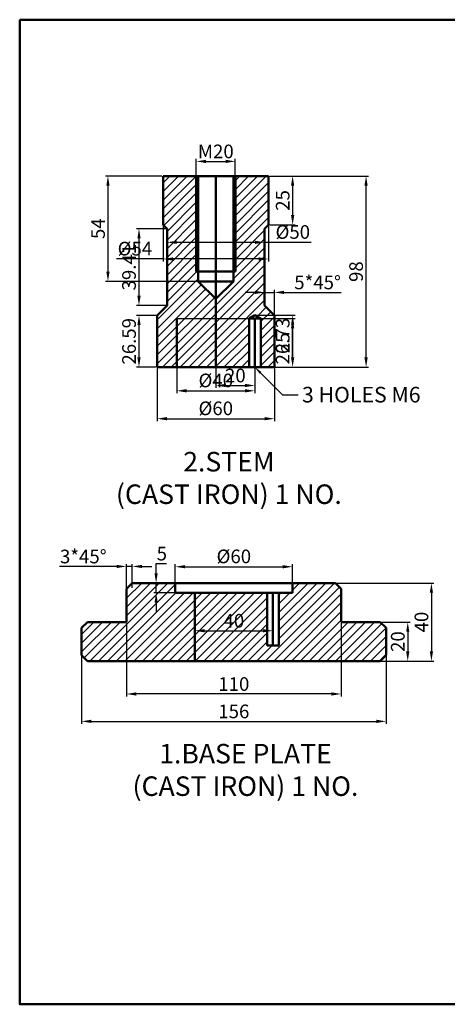
# Model space of a CAD drawing. Units: millimetres. Extents: x 51 to 972, y -225 to 280.
# Tile 1 of 3: x 51 to 270, y -225 to 280. Entities that reach past the tile are written whole.
import ezdxf
from ezdxf import colors
from ezdxf.entities.mleader import LeaderData, LeaderLine
from ezdxf.math import Vec2, Vec3

# ---------------------------------------------------------------- set-up
doc = ezdxf.new("R2010")
doc.units = ezdxf.units.MM
doc.header["$LTSCALE"] = 0.5
for name, color, linetype, lineweight in [('M-DIMS', 2, 'Continuous', 25), ('M-HATC', 8, 'Continuous', 18), ('M-OUTL', 7, 'Continuous', 50), ('M-TEXT', 7, 'Continuous', 25), ('M-TTLB', 7, 'Continuous', 50)]:
    doc.layers.add(name, color=color, linetype=linetype, lineweight=lineweight)
doc.styles.get("Standard").update_dxf_attribs({"font": 'arial.ttf'})
doc.dimstyles.new('ISO-25', dxfattribs={"dimtxt": 7, "dimasz": 5, "dimexe": 1.25, "dimexo": 0.625, "dimtad": 1, "dimtoh": 1, "dimtxsty": 'Standard', "dimcen": 2.5, "dimadec": 0, "dimazin": 0, "dimtfac": 1, "dimtmove": 0, "dimatfit": 3, "dimfxl": 1, "dimarcsym": 0})

# ---------------------------------------------------------------- blocks, each defined once
blk = doc.blocks.new('*D1')
at = {"layer": 'Defpoints', "color": 0, "transparency": 16777216}
for p in [(121.33, 101.59), (181.33, 101.59), (181.33, 75.2)]:
    blk.add_point(p, dxfattribs=at)
at = {"layer": 'M-DIMS', "color": 0, "lineweight": -2, "transparency": 16777216}
for p, q in [((121.33, 100.96), (121.33, 73.95)), ((181.33, 100.96), (181.33, 73.95)), ((126.33, 75.2), (176.33, 75.2))]:
    blk.add_line(p, q, dxfattribs=at)
at = {"layer": 'M-DIMS', "color": 0, "transparency": 16777216}
for points in [[(126.33, 76.04), (126.33, 74.37), (121.33, 75.2)], [(176.33, 76.04), (176.33, 74.37), (181.33, 75.2)]]:
    blk.add_solid(points, dxfattribs=at)
at = {"layer": 'M-DIMS', "color": 0, "transparency": 16777216, "insert": (151.33, 79.6), "char_height": 7, "attachment_point": 5}
blk.add_mtext('%%C60', dxfattribs=at)
blk = doc.blocks.new('*D2')
at = {"layer": 'Defpoints', "color": 0, "transparency": 16777216}
for p in [(131.33, 101.59), (171.33, 101.59), (171.33, 89.5)]:
    blk.add_point(p, dxfattribs=at)
at = {"layer": 'M-DIMS', "color": 0, "lineweight": -2, "transparency": 16777216}
for p, q in [((131.33, 100.96), (131.33, 88.25)), ((171.33, 100.96), (171.33, 88.25)), ((136.33, 89.5), (166.33, 89.5))]:
    blk.add_line(p, q, dxfattribs=at)
at = {"layer": 'M-DIMS', "color": 0, "transparency": 16777216}
for points in [[(136.33, 90.34), (136.33, 88.67), (131.33, 89.5)], [(166.33, 90.34), (166.33, 88.67), (171.33, 89.5)]]:
    blk.add_solid(points, dxfattribs=at)
at = {"layer": 'M-DIMS', "color": 0, "transparency": 16777216, "insert": (151.33, 93.9), "char_height": 7, "attachment_point": 5}
blk.add_mtext('%%C40', dxfattribs=at)
blk = doc.blocks.new('*D3')
at = {"layer": 'Defpoints', "color": 0, "transparency": 16777216}
for p in [(126.33, 168.2), (176.33, 168.2), (176.33, 165.61)]:
    blk.add_point(p, dxfattribs=at)
at = {"layer": 'M-DIMS', "color": 0, "lineweight": -2, "transparency": 16777216}
for p, q in [((126.33, 167.58), (126.33, 164.36)), ((176.33, 167.58), (176.33, 164.36)), ((131.33, 165.61), (171.33, 165.61)), ((176.33, 165.61), (200.2, 165.61))]:
    blk.add_line(p, q, dxfattribs=at)
at = {"layer": 'M-DIMS', "color": 0, "transparency": 16777216}
for points in [[(131.33, 166.44), (131.33, 164.77), (126.33, 165.61)], [(171.33, 166.44), (171.33, 164.77), (176.33, 165.61)]]:
    blk.add_solid(points, dxfattribs=at)
at = {"layer": 'M-DIMS', "color": 0, "transparency": 16777216, "insert": (190.77, 170), "char_height": 7, "attachment_point": 5}
blk.add_mtext('%%C50', dxfattribs=at)
blk = doc.blocks.new('*D4')
at = {"layer": 'Defpoints', "color": 0, "transparency": 16777216}
for p in [(124.33, 187.09), (178.33, 187.09), (178.33, 157.07)]:
    blk.add_point(p, dxfattribs=at)
at = {"layer": 'M-DIMS', "color": 0, "lineweight": -2, "transparency": 16777216}
for p, q in [((124.33, 186.46), (124.33, 155.82)), ((178.33, 186.46), (178.33, 155.82)), ((124.33, 157.07), (100.47, 157.07)), ((173.33, 157.07), (129.33, 157.07))]:
    blk.add_line(p, q, dxfattribs=at)
at = {"layer": 'M-DIMS', "color": 0, "transparency": 16777216}
for points in [[(129.33, 157.9), (129.33, 156.23), (124.33, 157.07)], [(173.33, 157.9), (173.33, 156.23), (178.33, 157.07)]]:
    blk.add_solid(points, dxfattribs=at)
at = {"layer": 'M-DIMS', "color": 0, "transparency": 16777216, "insert": (109.9, 161.46), "char_height": 7, "attachment_point": 5}
blk.add_mtext('%%C54', dxfattribs=at)
blk = doc.blocks.new('*D5')
at = {"layer": 'Defpoints', "color": 0, "transparency": 16777216}
for p in [(161.33, 207.09), (141.33, 199.59), (161.33, 199.59)]:
    blk.add_point(p, dxfattribs=at)
at = {"layer": 'M-DIMS', "color": 0, "lineweight": -2, "transparency": 16777216}
for p, q in [((141.33, 200.21), (141.33, 208.34)), ((146.33, 207.09), (156.33, 207.09)), ((161.33, 200.21), (161.33, 208.34))]:
    blk.add_line(p, q, dxfattribs=at)
at = {"layer": 'M-DIMS', "color": 0, "transparency": 16777216}
for points in [[(146.33, 207.92), (146.33, 206.25), (141.33, 207.09)], [(156.33, 207.92), (156.33, 206.25), (161.33, 207.09)]]:
    blk.add_solid(points, dxfattribs=at)
at = {"layer": 'M-DIMS', "color": 0, "transparency": 16777216, "insert": (151.33, 211.29), "char_height": 7, "attachment_point": 5}
blk.add_mtext('M20', dxfattribs=at)
blk = doc.blocks.new('*D6')
at = {"layer": 'Defpoints', "color": 0, "transparency": 16777216}
for p in [(181.33, 139.95), (176.33, 133.18), (181.33, 128.18)]:
    blk.add_point(p, dxfattribs=at)
at = {"layer": 'M-DIMS', "color": 0, "lineweight": -2, "transparency": 16777216}
for p, q in [((171.33, 139.95), (166.33, 139.95)), ((176.33, 133.8), (176.33, 141.2)), ((176.33, 139.95), (181.33, 139.95)), ((181.33, 128.8), (181.33, 141.2)), ((186.33, 139.95), (215.56, 139.95))]:
    blk.add_line(p, q, dxfattribs=at)
at = {"layer": 'M-DIMS', "color": 0, "transparency": 16777216}
for points in [[(171.33, 140.78), (171.33, 139.12), (176.33, 139.95)], [(186.33, 140.78), (186.33, 139.12), (181.33, 139.95)]]:
    blk.add_solid(points, dxfattribs=at)
at = {"layer": 'M-DIMS', "color": 0, "transparency": 16777216, "insert": (203.45, 144.14), "char_height": 7, "attachment_point": 5}
blk.add_mtext('5*45%%D', dxfattribs=at)
blk = doc.blocks.new('*D7')
at = {"layer": 'Defpoints', "color": 0, "transparency": 16777216}
for p in [(178.33, 199.59), (228.3, 199.59), (181.45, 101.59)]:
    blk.add_point(p, dxfattribs=at)
at = {"layer": 'M-DIMS', "color": 0, "lineweight": -2, "transparency": 16777216}
for p, q in [((178.96, 199.59), (229.55, 199.59)), ((228.3, 106.59), (228.3, 194.59)), ((182.08, 101.59), (229.55, 101.59))]:
    blk.add_line(p, q, dxfattribs=at)
at = {"layer": 'M-DIMS', "color": 0, "transparency": 16777216}
for points in [[(227.46, 194.59), (229.13, 194.59), (228.3, 199.59)], [(227.46, 106.59), (229.13, 106.59), (228.3, 101.59)]]:
    blk.add_solid(points, dxfattribs=at)
at = {"layer": 'M-DIMS', "color": 0, "transparency": 16777216, "insert": (224.1, 150.59), "char_height": 7, "attachment_point": 5, "rotation": 90}
blk.add_mtext('98', dxfattribs=at)
blk = doc.blocks.new('*D8')
at = {"layer": 'Defpoints', "color": 0, "transparency": 16777216}
for p in [(124.33, 199.59), (96.09, 145.59), (151.33, 145.59)]:
    blk.add_point(p, dxfattribs=at)
at = {"layer": 'M-DIMS', "color": 0, "lineweight": -2, "transparency": 16777216}
for p, q in [((123.71, 199.59), (94.84, 199.59)), ((96.09, 194.59), (96.09, 150.59)), ((150.71, 145.59), (94.84, 145.59))]:
    blk.add_line(p, q, dxfattribs=at)
at = {"layer": 'M-DIMS', "color": 0, "transparency": 16777216}
for points in [[(95.26, 194.59), (96.93, 194.59), (96.09, 199.59)], [(95.26, 150.59), (96.93, 150.59), (96.09, 145.59)]]:
    blk.add_solid(points, dxfattribs=at)
at = {"layer": 'M-DIMS', "color": 0, "transparency": 16777216, "insert": (91.91, 172.59), "char_height": 7, "attachment_point": 5, "rotation": 90}
blk.add_mtext('54', dxfattribs=at)
blk = doc.blocks.new('*D20')
at = {"layer": 'Defpoints', "color": 0, "ltscale": 0.5, "transparency": 16777216}
for p in [(82.57, -39.05), (238.57, -39.05), (238.57, -79.94)]:
    blk.add_point(p, dxfattribs=at)
at = {"layer": 'M-DIMS', "color": 0, "lineweight": -2, "ltscale": 0.5, "transparency": 16777216}
for p, q in [((82.57, -39.67), (82.57, -81.19)), ((238.57, -39.67), (238.57, -81.19)), ((87.57, -79.94), (233.57, -79.94))]:
    blk.add_line(p, q, dxfattribs=at)
at = {"layer": 'M-DIMS', "color": 0, "ltscale": 0.5, "transparency": 16777216}
for points in [[(87.57, -79.1), (87.57, -80.77), (82.57, -79.94)], [(233.57, -79.1), (233.57, -80.77), (238.57, -79.94)]]:
    blk.add_solid(points, dxfattribs=at)
at = {"layer": 'M-DIMS', "color": 0, "ltscale": 0.5, "transparency": 16777216, "insert": (160.57, -75.74), "char_height": 7, "attachment_point": 5}
blk.add_mtext('156', dxfattribs=at)
blk = doc.blocks.new('*D21')
at = {"layer": 'Defpoints', "color": 0, "ltscale": 0.5, "transparency": 16777216}
for p in [(105.57, -29.05), (215.57, -29.05), (105.57, -65.91)]:
    blk.add_point(p, dxfattribs=at)
at = {"layer": 'M-DIMS', "color": 0, "lineweight": -2, "ltscale": 0.5, "transparency": 16777216}
for p, q in [((105.57, -29.67), (105.57, -67.16)), ((215.57, -29.67), (215.57, -67.16)), ((210.57, -65.91), (110.57, -65.91))]:
    blk.add_line(p, q, dxfattribs=at)
at = {"layer": 'M-DIMS', "color": 0, "ltscale": 0.5, "transparency": 16777216}
for points in [[(110.57, -65.07), (110.57, -66.74), (105.57, -65.91)], [(210.57, -65.07), (210.57, -66.74), (215.57, -65.91)]]:
    blk.add_solid(points, dxfattribs=at)
at = {"layer": 'M-DIMS', "color": 0, "ltscale": 0.5, "transparency": 16777216, "insert": (160.57, -61.71), "char_height": 7, "attachment_point": 5}
blk.add_mtext('110', dxfattribs=at)
blk = doc.blocks.new('*D22')
at = {"layer": 'Defpoints', "color": 0, "ltscale": 0.5, "transparency": 16777216}
for p in [(190.57, -0.69), (130.57, -9.05), (190.57, -9.05)]:
    blk.add_point(p, dxfattribs=at)
at = {"layer": 'M-DIMS', "color": 0, "lineweight": -2, "ltscale": 0.5, "transparency": 16777216}
for p, q in [((130.57, -8.42), (130.57, 0.56)), ((190.57, -8.42), (190.57, 0.56)), ((135.57, -0.69), (185.57, -0.69))]:
    blk.add_line(p, q, dxfattribs=at)
at = {"layer": 'M-DIMS', "color": 0, "ltscale": 0.5, "transparency": 16777216}
for points in [[(135.57, 0.14), (135.57, -1.52), (130.57, -0.69)], [(185.57, 0.14), (185.57, -1.52), (190.57, -0.69)]]:
    blk.add_solid(points, dxfattribs=at)
at = {"layer": 'M-DIMS', "color": 0, "ltscale": 0.5, "transparency": 16777216, "insert": (160.57, 3.71), "char_height": 7, "attachment_point": 5}
blk.add_mtext('%%C60', dxfattribs=at)
blk = doc.blocks.new('*D23')
at = {"layer": 'Defpoints', "color": 0, "ltscale": 0.5, "transparency": 16777216}
for p in [(140.57, -31.55), (180.57, -31.55), (180.57, -33.49)]:
    blk.add_point(p, dxfattribs=at)
at = {"layer": 'M-DIMS', "color": 0, "lineweight": -2, "ltscale": 0.5, "transparency": 16777216}
for p, q in [((140.57, -32.17), (140.57, -34.74)), ((145.57, -33.49), (175.57, -33.49)), ((180.57, -32.17), (180.57, -34.74))]:
    blk.add_line(p, q, dxfattribs=at)
at = {"layer": 'M-DIMS', "color": 0, "ltscale": 0.5, "transparency": 16777216}
for points in [[(145.57, -32.66), (145.57, -34.33), (140.57, -33.49)], [(175.57, -32.66), (175.57, -34.33), (180.57, -33.49)]]:
    blk.add_solid(points, dxfattribs=at)
at = {"layer": 'M-DIMS', "color": 0, "ltscale": 0.5, "transparency": 16777216, "insert": (160.57, -29.29), "char_height": 7, "attachment_point": 5}
blk.add_mtext('40', dxfattribs=at)
blk = doc.blocks.new('*D24')
at = {"layer": 'Defpoints', "color": 0, "ltscale": 0.5, "transparency": 16777216}
for p in [(130.57, -9.05), (120.76, -14.05), (130.57, -14.05)]:
    blk.add_point(p, dxfattribs=at)
at = {"layer": 'M-DIMS', "color": 0, "lineweight": -2, "ltscale": 0.5, "transparency": 16777216}
for p, q in [((120.76, -4.05), (120.76, 0.95)), ((120.76, 0.95), (126.03, 0.95)), ((129.94, -9.05), (119.51, -9.05)), ((120.76, -14.05), (120.76, -9.05)), ((129.94, -14.05), (119.51, -14.05)), ((120.76, -19.05), (120.76, -24.05))]:
    blk.add_line(p, q, dxfattribs=at)
at = {"layer": 'M-DIMS', "color": 0, "ltscale": 0.5, "transparency": 16777216}
for points in [[(119.93, -4.05), (121.59, -4.05), (120.76, -9.05)], [(119.93, -19.05), (121.59, -19.05), (120.76, -14.05)]]:
    blk.add_solid(points, dxfattribs=at)
at = {"layer": 'M-DIMS', "color": 0, "ltscale": 0.5, "transparency": 16777216, "insert": (123.7, 5.14), "char_height": 7, "attachment_point": 5}
blk.add_mtext('5', dxfattribs=at)
blk = doc.blocks.new('*D25')
at = {"layer": 'Defpoints', "color": 0, "ltscale": 0.5, "transparency": 16777216}
for p in [(108.57, -0.54), (105.57, -12.05), (108.57, -12.05)]:
    blk.add_point(p, dxfattribs=at)
at = {"layer": 'M-DIMS', "color": 0, "lineweight": -2, "ltscale": 0.5, "transparency": 16777216}
for p, q in [((105.57, -11.42), (105.57, 0.71)), ((108.57, -11.42), (108.57, 0.71)), ((100.57, -0.54), (71.35, -0.54)), ((108.57, -0.54), (105.57, -0.54)), ((113.57, -0.54), (118.57, -0.54))]:
    blk.add_line(p, q, dxfattribs=at)
at = {"layer": 'M-DIMS', "color": 0, "ltscale": 0.5, "transparency": 16777216}
for points in [[(100.57, 0.29), (100.57, -1.37), (105.57, -0.54)], [(113.57, 0.29), (113.57, -1.37), (108.57, -0.54)]]:
    blk.add_solid(points, dxfattribs=at)
at = {"layer": 'M-DIMS', "color": 0, "ltscale": 0.5, "transparency": 16777216, "insert": (83.46, 3.66), "char_height": 7, "attachment_point": 5}
blk.add_mtext('3*45%%D', dxfattribs=at)
blk = doc.blocks.new('*D26')
at = {"layer": 'Defpoints', "color": 0, "ltscale": 0.5, "transparency": 16777216}
for p in [(210, -9.05), (207.19, -49.05), (261.77, -49.05)]:
    blk.add_point(p, dxfattribs=at)
at = {"layer": 'M-DIMS', "color": 0, "lineweight": -2, "ltscale": 0.5, "transparency": 16777216}
for p, q in [((210.63, -9.05), (263.02, -9.05)), ((261.77, -14.05), (261.77, -44.05)), ((207.82, -49.05), (263.02, -49.05))]:
    blk.add_line(p, q, dxfattribs=at)
at = {"layer": 'M-DIMS', "color": 0, "ltscale": 0.5, "transparency": 16777216}
for points in [[(260.93, -14.05), (262.6, -14.05), (261.77, -9.05)], [(260.93, -44.05), (262.6, -44.05), (261.77, -49.05)]]:
    blk.add_solid(points, dxfattribs=at)
at = {"layer": 'M-DIMS', "color": 0, "ltscale": 0.5, "transparency": 16777216, "insert": (257.57, -29.05), "char_height": 7, "attachment_point": 5, "rotation": 90}
blk.add_mtext('40', dxfattribs=at)
blk = doc.blocks.new('*D27')
at = {"layer": 'Defpoints', "color": 0, "ltscale": 0.5, "transparency": 16777216}
for p in [(232.48, -29.05), (232.48, -49.05), (249.65, -49.05)]:
    blk.add_point(p, dxfattribs=at)
at = {"layer": 'M-DIMS', "color": 0, "lineweight": -2, "ltscale": 0.5, "transparency": 16777216}
for p, q in [((233.11, -29.05), (250.9, -29.05)), ((249.65, -34.05), (249.65, -44.05)), ((233.11, -49.05), (250.9, -49.05))]:
    blk.add_line(p, q, dxfattribs=at)
at = {"layer": 'M-DIMS', "color": 0, "ltscale": 0.5, "transparency": 16777216}
for points in [[(248.82, -34.05), (250.48, -34.05), (249.65, -29.05)], [(248.82, -44.05), (250.48, -44.05), (249.65, -49.05)]]:
    blk.add_solid(points, dxfattribs=at)
at = {"layer": 'M-DIMS', "color": 0, "ltscale": 0.5, "transparency": 16777216, "insert": (245.45, -39.05), "char_height": 7, "attachment_point": 5, "rotation": 90}
blk.add_mtext('20', dxfattribs=at)
blk = doc.blocks.new('*D52')
at = {"layer": 'Defpoints', "color": 0, "ltscale": 0.5, "transparency": 16777216}
for p in [(178.33, 199.59), (178.33, 174.59), (190.68, 174.59)]:
    blk.add_point(p, dxfattribs=at)
at = {"layer": 'M-DIMS', "color": 0, "lineweight": -2, "ltscale": 0.5, "transparency": 16777216}
for p, q in [((178.96, 199.59), (191.93, 199.59)), ((190.68, 194.59), (190.68, 179.59)), ((178.96, 174.59), (191.93, 174.59))]:
    blk.add_line(p, q, dxfattribs=at)
at = {"layer": 'M-DIMS', "color": 0, "ltscale": 0.5, "transparency": 16777216}
for points in [[(189.85, 194.59), (191.52, 194.59), (190.68, 199.59)], [(189.85, 179.59), (191.52, 179.59), (190.68, 174.59)]]:
    blk.add_solid(points, dxfattribs=at)
at = {"layer": 'M-DIMS', "color": 0, "ltscale": 0.5, "transparency": 16777216, "insert": (186.49, 187.09), "char_height": 7, "attachment_point": 5, "rotation": 90}
blk.add_mtext('25', dxfattribs=at)
blk = doc.blocks.new('*D53')
at = {"layer": 'Defpoints', "color": 0, "ltscale": 0.5, "transparency": 16777216}
for p in [(126.33, 172.59), (111.98, 133.18), (126.33, 133.18)]:
    blk.add_point(p, dxfattribs=at)
at = {"layer": 'M-DIMS', "color": 0, "lineweight": -2, "ltscale": 0.5, "transparency": 16777216}
for p, q in [((125.71, 172.59), (110.73, 172.59)), ((111.98, 167.59), (111.98, 138.18)), ((125.71, 133.18), (110.73, 133.18))]:
    blk.add_line(p, q, dxfattribs=at)
at = {"layer": 'M-DIMS', "color": 0, "ltscale": 0.5, "transparency": 16777216}
for points in [[(111.15, 167.59), (112.82, 167.59), (111.98, 172.59)], [(111.15, 138.18), (112.82, 138.18), (111.98, 133.18)]]:
    blk.add_solid(points, dxfattribs=at)
at = {"layer": 'M-DIMS', "color": 0, "ltscale": 0.5, "transparency": 16777216, "insert": (107.78, 152.88), "char_height": 7, "attachment_point": 5, "rotation": 90}
blk.add_mtext('39.41', dxfattribs=at)
blk = doc.blocks.new('*D54')
at = {"layer": 'Defpoints', "color": 0, "ltscale": 0.5, "transparency": 16777216}
for p in [(121.33, 128.18), (111.98, 101.59), (121.33, 101.59)]:
    blk.add_point(p, dxfattribs=at)
at = {"layer": 'M-DIMS', "color": 0, "lineweight": -2, "ltscale": 0.5, "transparency": 16777216}
for p, q in [((120.71, 128.18), (110.73, 128.18)), ((111.98, 123.18), (111.98, 106.59)), ((120.71, 101.59), (110.73, 101.59))]:
    blk.add_line(p, q, dxfattribs=at)
at = {"layer": 'M-DIMS', "color": 0, "ltscale": 0.5, "transparency": 16777216}
for points in [[(111.15, 123.18), (112.82, 123.18), (111.98, 128.18)], [(111.15, 106.59), (112.82, 106.59), (111.98, 101.59)]]:
    blk.add_solid(points, dxfattribs=at)
at = {"layer": 'M-DIMS', "color": 0, "ltscale": 0.5, "transparency": 16777216, "insert": (107.79, 114.88), "char_height": 7, "attachment_point": 5, "rotation": 90}
blk.add_mtext('26.59', dxfattribs=at)
blk = doc.blocks.new('*D55')
at = {"layer": 'Defpoints', "color": 0, "ltscale": 0.5, "transparency": 16777216}
for p in [(131.33, 126.59), (190.68, 126.59), (131.33, 101.59)]:
    blk.add_point(p, dxfattribs=at)
at = {"layer": 'M-DIMS', "color": 0, "lineweight": -2, "ltscale": 0.5, "transparency": 16777216}
for p, q in [((131.96, 126.59), (191.93, 126.59)), ((190.68, 106.59), (190.68, 121.59)), ((131.96, 101.59), (191.93, 101.59))]:
    blk.add_line(p, q, dxfattribs=at)
at = {"layer": 'M-DIMS', "color": 0, "ltscale": 0.5, "transparency": 16777216}
for points in [[(189.85, 121.59), (191.52, 121.59), (190.68, 126.59)], [(189.85, 106.59), (191.52, 106.59), (190.68, 101.59)]]:
    blk.add_solid(points, dxfattribs=at)
at = {"layer": 'M-DIMS', "color": 0, "ltscale": 0.5, "transparency": 16777216, "insert": (186.49, 114.09), "char_height": 7, "attachment_point": 5, "rotation": 90}
blk.add_mtext('25', dxfattribs=at)
blk = doc.blocks.new('*D56')
at = {"layer": 'Defpoints', "color": 0, "ltscale": 0.5, "transparency": 16777216}
for p in [(171.33, 128.32), (171.33, 101.59), (190.68, 101.59)]:
    blk.add_point(p, dxfattribs=at)
at = {"layer": 'M-DIMS', "color": 0, "lineweight": -2, "ltscale": 0.5, "transparency": 16777216}
for p, q in [((171.96, 128.32), (191.93, 128.32)), ((190.68, 123.32), (190.68, 106.59)), ((171.96, 101.59), (191.93, 101.59))]:
    blk.add_line(p, q, dxfattribs=at)
at = {"layer": 'M-DIMS', "color": 0, "ltscale": 0.5, "transparency": 16777216}
for points in [[(189.85, 123.32), (191.52, 123.32), (190.68, 128.32)], [(189.85, 106.59), (191.52, 106.59), (190.68, 101.59)]]:
    blk.add_solid(points, dxfattribs=at)
at = {"layer": 'M-DIMS', "color": 0, "ltscale": 0.5, "transparency": 16777216, "insert": (186.48, 114.95), "char_height": 7, "attachment_point": 5, "rotation": 90}
blk.add_mtext('26.73', dxfattribs=at)
blk = doc.blocks.new('*D57')
at = {"layer": 'Defpoints', "color": 0, "ltscale": 0.5, "transparency": 16777216}
for p in [(151.33, 101.59), (171.33, 101.59), (171.33, 92.24)]:
    blk.add_point(p, dxfattribs=at)
at = {"layer": 'M-DIMS', "color": 0, "lineweight": -2, "ltscale": 0.5, "transparency": 16777216}
for p, q in [((151.33, 100.96), (151.33, 90.99)), ((171.33, 100.96), (171.33, 90.99)), ((156.33, 92.24), (166.33, 92.24))]:
    blk.add_line(p, q, dxfattribs=at)
at = {"layer": 'M-DIMS', "color": 0, "ltscale": 0.5, "transparency": 16777216}
for points in [[(156.33, 93.07), (156.33, 91.4), (151.33, 92.24)], [(166.33, 93.07), (166.33, 91.4), (171.33, 92.24)]]:
    blk.add_solid(points, dxfattribs=at)
at = {"layer": 'M-DIMS', "color": 0, "ltscale": 0.5, "transparency": 16777216, "insert": (161.33, 96.44), "char_height": 7, "attachment_point": 5}
blk.add_mtext('20', dxfattribs=at)

msp = doc.modelspace()

# ---------------------------------------------------------------- hatches: boundary and pattern name
at = {"layer": 'M-HATC'}
h = msp.add_hatch(dxfattribs=at)
h.set_pattern_fill('ANSI31', color=256)
h.paths.add_polyline_path([(141.3347, 199.5882), (126.3347, 199.5882), (124.3347, 199.5882), (124.3347, 174.5882), (126.3347, 172.5882), (126.3347, 133.1786), (121.3347, 128.1786), (121.3347, 101.5882), (151.3347, 101.5882), (151.3347, 136.5882), (142.3347, 145.5882), (142.3347, 150.5882), (141.3347, 150.5882)])
h.paths.add_polyline_path([(178.3347, 199.5882), (161.3347, 199.5882), (161.3347, 150.5882), (160.3347, 150.5882), (160.3347, 145.5882), (151.3347, 136.5882), (151.3347, 101.5882), (168.3347, 101.5882), (168.3347, 126.5882), (171.3347, 128.3202), (174.3347, 126.5882), (174.3347, 101.5882), (181.3347, 101.5882), (181.3347, 128.1786), (176.3347, 133.1786), (176.3347, 172.5882), (178.3347, 174.5882)])
at = {"layer": 'M-HATC', "ltscale": 0.5}
h = msp.add_hatch(dxfattribs=at)
h.set_pattern_fill('ANSI31', color=256)
h.set_pattern_definition([(45, (-465.4576, -116.4076), (-2.245064, 2.245064), [])])
h.paths.add_polyline_path([(140.5681, -14.0451), (130.5681, -14.0451), (130.5681, -9.0451), (108.5681, -9.0451), (105.5681, -12.0451), (105.5681, -29.0451), (85.5681, -29.0451), (82.5681, -32.0451), (82.5681, -46.0451), (85.5681, -49.0451), (140.5681, -49.0451)])
h.paths.add_polyline_path([(238.5681, -32.0451), (235.5681, -29.0451), (215.5681, -29.0451), (215.5681, -12.0451), (212.5681, -9.0451), (190.5681, -9.0451), (190.5681, -14.0451), (183.5681, -14.0451), (183.5681, -41.0451), (177.5681, -41.0451), (177.5681, -14.0451), (140.5681, -14.0451), (140.5681, -49.0451), (235.5681, -49.0451), (238.5681, -46.0451)])
h.paths.add_polyline_path([(153.5514, -36.57), (167.9286, -36.57), (167.9286, -22.145), (153.5514, -22.145)], flags=24)

# ---------------------------------------------------------------- linework, layer by layer
at = {"layer": 'M-OUTL'}
for p, q in [((124.3347, 174.5882), (124.3347, 199.5882)), ((124.3347, 199.5882), (126.3347, 199.5882)), ((176.3347, 199.5882), (126.3347, 199.5882)), ((141.3347, 150.5882), (141.3347, 199.5882)), ((142.3347, 145.5882), (142.3347, 199.5882)), ((151.3347, 199.5882), (151.3347, 101.5882)), ((151.3347, 199.5882), (178.3347, 199.5882)), ((160.3347, 199.5882), (160.3347, 145.5882)), ((161.3347, 199.5882), (161.3347, 150.5882)), ((178.3347, 199.5882), (178.3347, 174.5882)), ((124.3347, 174.5882), (126.3347, 172.5882)), ((126.3347, 133.1786), (126.3347, 172.5882)), ((178.3347, 174.5882), (176.3347, 172.5882)), ((176.3347, 172.5882), (176.3347, 133.1786)), ((161.3347, 150.5882), (141.3347, 150.5882)), ((160.3347, 145.5882), (142.3347, 145.5882)), ((142.3347, 145.5882), (151.3347, 136.5882)), ((160.3347, 145.5882), (151.3347, 136.5882)), ((121.3347, 128.1786), (126.3347, 133.1786)), ((181.3347, 128.1786), (176.3347, 133.1786)), ((121.3347, 128.1786), (121.3347, 101.5882)), ((131.3347, 126.5882), (131.3347, 101.5882)), ((168.3347, 126.5882), (171.3347, 128.3202)), ((168.3347, 126.5882), (168.3347, 101.5882)), ((168.3347, 126.5882), (174.3347, 126.5882)), ((174.3347, 126.5882), (171.3347, 128.3202)), ((171.3347, 126.5882), (171.3347, 101.5882)), ((174.3347, 126.5882), (174.3347, 101.5882)), ((181.3347, 101.5882), (181.3347, 128.1786)), ((121.3347, 101.5882), (181.3347, 101.5882))]:
    msp.add_line(p, q, dxfattribs=at)
at = {"layer": 'M-OUTL', "ltscale": 0.5}
for p, q in [((108.5681, -9.0451), (105.5681, -12.0451)), ((212.5681, -9.0451), (108.5681, -9.0451)), ((130.5681, -14.0451), (130.5681, -9.0451)), ((190.5681, -9.0451), (190.5681, -14.0451)), ((212.5681, -9.0451), (215.5681, -12.0451)), ((105.5681, -12.0451), (105.5681, -29.0451)), ((190.5681, -14.0451), (130.5681, -14.0451)), ((140.5681, -14.0451), (140.5681, -49.0451)), ((177.5681, -14.0451), (177.5681, -41.0451)), ((180.5681, -14.0451), (180.5681, -41.0451)), ((183.5681, -14.0451), (183.5681, -41.0451)), ((215.5681, -29.0451), (215.5681, -12.0451)), ((85.5681, -29.0451), (82.5681, -32.0451)), ((105.5681, -29.0451), (85.5681, -29.0451)), ((235.5681, -29.0451), (215.5681, -29.0451)), ((235.5681, -29.0451), (238.5681, -32.0451)), ((82.5681, -32.0451), (82.5681, -46.0451)), ((238.5681, -46.0451), (238.5681, -32.0451)), ((177.5681, -41.0451), (183.5681, -41.0451)), ((82.5681, -46.0451), (85.5681, -49.0451)), ((85.5681, -49.0451), (235.5681, -49.0451)), ((238.5681, -46.0451), (235.5681, -49.0451))]:
    msp.add_line(p, q, dxfattribs=at)
at = {"layer": 'M-TTLB', "ltscale": 0.5}
msp.add_lwpolyline([(50.8898, 279.7282), (925.0778, 279.7282), (925.0778, -224.9845), (50.8898, -224.9845)], close=True, dxfattribs=at)

# ---------------------------------------------------------------- texts
at = {"layer": 'M-TEXT', "char_height": 10, "attachment_point": 1}
for s, insert in [('\\pxqc;2.STEM \\P(CAST IRON) 1 NO. ', (62.3177, 58.155)), ('\\pxqc;1.BASE PLATE \\P(CAST IRON) 1 NO. ', (70.8111, -91.498))]:
    msp.add_mtext_dynamic_manual_height_columns(s, width=191.418549, gutter_width=12.5, heights=[0], dxfattribs=dict(at, insert=insert))

# ---------------------------------------------------------------- dimensions: what is measured, and where the dimension line sits
at = {"layer": 'M-DIMS'}
for base, p1, p2, text, picture, middle in [((161.3347, 207.0883), (141.3347, 199.5882), (161.3347, 199.5882), 'M<>', '*D5', (151.3347, 211.2873)), ((181.3347, 139.9504), (176.3347, 133.1786), (181.3347, 128.1786), '<>*45%%D', '*D6', (203.4481, 144.1351))]:
    dim = msp.add_linear_dim(base=base, p1=p1, p2=p2, text=text, dimstyle='ISO-25', override={"dimclrd": 0, "dimclre": 0, "dimclrt": 0}, dxfattribs=at)
    dim.commit()
    dim.dimension.update_dxf_attribs({"geometry": picture, "text_midpoint": middle})
for base, p1, p2, picture, middle in [((96.0917, 145.5882), (124.3347, 199.5882), (151.3347, 145.5882), '*D8', (91.907, 172.5882)), ((228.2957, 199.5882), (181.4518, 101.5882), (178.3347, 199.5882), '*D7', (224.0967, 150.5882))]:
    dim = msp.add_linear_dim(base=base, p1=p1, p2=p2, angle=90, dimstyle='ISO-25', override={"dimclrd": 0, "dimclre": 0, "dimclrt": 0}, dxfattribs=at)
    dim.commit()
    dim.dimension.update_dxf_attribs({"geometry": picture, "text_midpoint": middle})
at = {"layer": 'M-DIMS', "ltscale": 0.5}
for base, p1, p2, override, picture, middle in [((190.6847, 174.5882), (178.3347, 199.5882), (178.3347, 174.5882), {"dimdec": 0, "dimlfac": 1, "dimrnd": 0, "dimzin": 0, "dimdsep": 46, "dimlunit": 2}, '*D52', (186.4857, 187.0882)), ((111.9847, 133.1786), (126.3347, 172.5882), (126.3347, 133.1786), {"dimdec": 2, "dimlfac": 1, "dimrnd": 0, "dimzin": 0, "dimdsep": 46, "dimlunit": 2}, '*D53', (107.7833, 152.8834)), ((111.9847, 101.5882), (121.3347, 128.1786), (121.3347, 101.5882), {"dimdec": 2, "dimlfac": 1, "dimrnd": 0, "dimzin": 0, "dimdsep": 46, "dimlunit": 2}, '*D54', (107.7857, 114.8834)), ((190.6847, 126.5882), (131.3347, 101.5882), (131.3347, 126.5882), {"dimdec": 0, "dimlfac": 1, "dimrnd": 0, "dimzin": 0, "dimdsep": 46, "dimlunit": 2}, '*D55', (186.4857, 114.0882)), ((190.6847, 101.5882), (171.3347, 128.3202), (171.3347, 101.5882), {"dimdec": 2, "dimlfac": 1, "dimrnd": 0, "dimzin": 0, "dimdsep": 46, "dimlunit": 2}, '*D56', (186.4833, 114.9542)), ((261.7659, -49.0451), (210.0049, -9.0451), (207.1933, -49.0451), {"dimclrd": 0, "dimclre": 0, "dimclrt": 0}, '*D26', (257.5669, -29.0451)), ((249.6493, -49.0451), (232.484, -29.0451), (232.484, -49.0451), {"dimclrd": 0, "dimclre": 0, "dimclrt": 0}, '*D27', (245.4502, -39.0451))]:
    dim = msp.add_linear_dim(base=base, p1=p1, p2=p2, angle=90, dimstyle='ISO-25', override=override, dxfattribs=at)
    dim.commit()
    dim.dimension.update_dxf_attribs({"geometry": picture, "text_midpoint": middle})
at = {"layer": 'M-DIMS'}
for base, p1, p2, picture, middle in [((178.3347, 157.068), (124.3347, 187.0882), (178.3347, 187.0882), '*D4', (109.9024, 157.068)), ((176.3347, 165.6077), (126.3347, 168.2018), (176.3347, 168.2018), '*D3', (190.7694, 165.6077)), ((181.3347, 75.2033), (121.3347, 101.5882), (181.3347, 101.5882), '*D1', (151.3347, 75.2033)), ((171.3347, 89.5026), (131.3347, 101.5882), (171.3347, 101.5882), '*D2', (151.3347, 89.5026))]:
    dim = msp.add_linear_dim(base=base, p1=p1, p2=p2, text='%%C<>', dimstyle='ISO-25', override={"dimclrd": 0, "dimclre": 0, "dimclrt": 0}, dxfattribs=at)
    dim.commit()
    dim.dimension.update_dxf_attribs({"geometry": picture, "text_midpoint": middle, "dimtype": 160})
at = {"layer": 'M-DIMS', "ltscale": 0.5}
for base, p1, p2, override, picture, middle in [((171.3347, 92.2382), (151.3347, 101.5882), (171.3347, 101.5882), {"dimdec": 0, "dimlfac": 1, "dimrnd": 0, "dimzin": 0, "dimdsep": 46, "dimlunit": 2}, '*D57', (161.3347, 96.4372)), ((180.5681, -33.4921), (140.5681, -31.5451), (180.5681, -31.5451), {"dimclrd": 0, "dimclre": 0, "dimclrt": 0}, '*D23', (160.5681, -29.2931)), ((105.5681, -65.9065), (215.5681, -29.0451), (105.5681, -29.0451), {"dimclrd": 0, "dimclre": 0, "dimclrt": 0}, '*D21', (160.5681, -61.7075)), ((238.5681, -79.9375), (82.5681, -39.0451), (238.5681, -39.0451), {"dimclrd": 0, "dimclre": 0, "dimclrt": 0}, '*D20', (160.5681, -75.7385))]:
    dim = msp.add_linear_dim(base=base, p1=p1, p2=p2, dimstyle='ISO-25', override=override, dxfattribs=at)
    dim.commit()
    dim.dimension.update_dxf_attribs({"geometry": picture, "text_midpoint": middle})
dim = msp.add_linear_dim(base=(108.5681, -0.5411), p1=(105.5681, -12.0451), p2=(108.5681, -12.0451), text='<>*45%%D', dimstyle='ISO-25', override={"dimclrd": 0, "dimclre": 0, "dimclrt": 0}, dxfattribs=at)
dim.commit()
dim.dimension.update_dxf_attribs({"geometry": '*D25', "text_midpoint": (83.4571, -0.5411), "dimtype": 160})
dim = msp.add_linear_dim(base=(120.7592, -14.0451), p1=(130.5681, -9.0451), p2=(130.5681, -14.0451), angle=90, dimstyle='ISO-25', override={"dimclrd": 0, "dimclre": 0, "dimclrt": 0}, dxfattribs=at)
dim.commit()
dim.dimension.update_dxf_attribs({"geometry": '*D24', "text_midpoint": (123.7048, 0.9549), "dimtype": 160})
dim = msp.add_linear_dim(base=(190.5681, -0.6894), p1=(130.5681, -9.0451), p2=(190.5681, -9.0451), text='%%C<>', dimstyle='ISO-25', override={"dimclrd": 0, "dimclre": 0, "dimclrt": 0}, dxfattribs=at)
dim.commit()
dim.dimension.update_dxf_attribs({"geometry": '*D22', "text_midpoint": (160.5681, 3.7054)})

# ---------------------------------------------------------------- leaders
at = {"layer": 'M-DIMS'}
ml = msp.add_multileader_mtext('Standard', dxfattribs=at)
ml.set_content('3 HOLES M6', color=256)
ml.set_leader_properties()
ml.build(insert=Vec2(0, 0))
ctx = ml.context
ctx.base_point, ctx.char_height, ctx.plane_origin = Vec3(193.4647, 87.4582), 8, Vec3(171.3347, 101.5882)
notes = []
notes.append((ctx, [(0, (1, 1, 0), (185.4647, 87.4582), (1, 0), 8, [(0, [(171.3347, 101.5882)], 0, [])])]))
ctx.mtext.insert, ctx.mtext.flow_direction = Vec3(195.4647, 91.5292), 5
for ctx, leaders in notes:
    for number, flags, end, landing, length, lines in leaders:
        leader = LeaderData()
        leader.index, (leader.has_last_leader_line, leader.has_dogleg_vector, leader.attachment_direction) = number, flags
        leader.last_leader_point, leader.dogleg_vector, leader.dogleg_length = Vec3(end), Vec3(landing), length
        for number, points, colour, breaks in lines:
            line = LeaderLine()
            line.index, line.vertices, line.color, line.breaks = number, Vec3.list(points), colors.encode_raw_color(colour), breaks
            leader.lines.append(line)
        ctx.leaders.append(leader)

doc.saveas('drawing.dxf')
